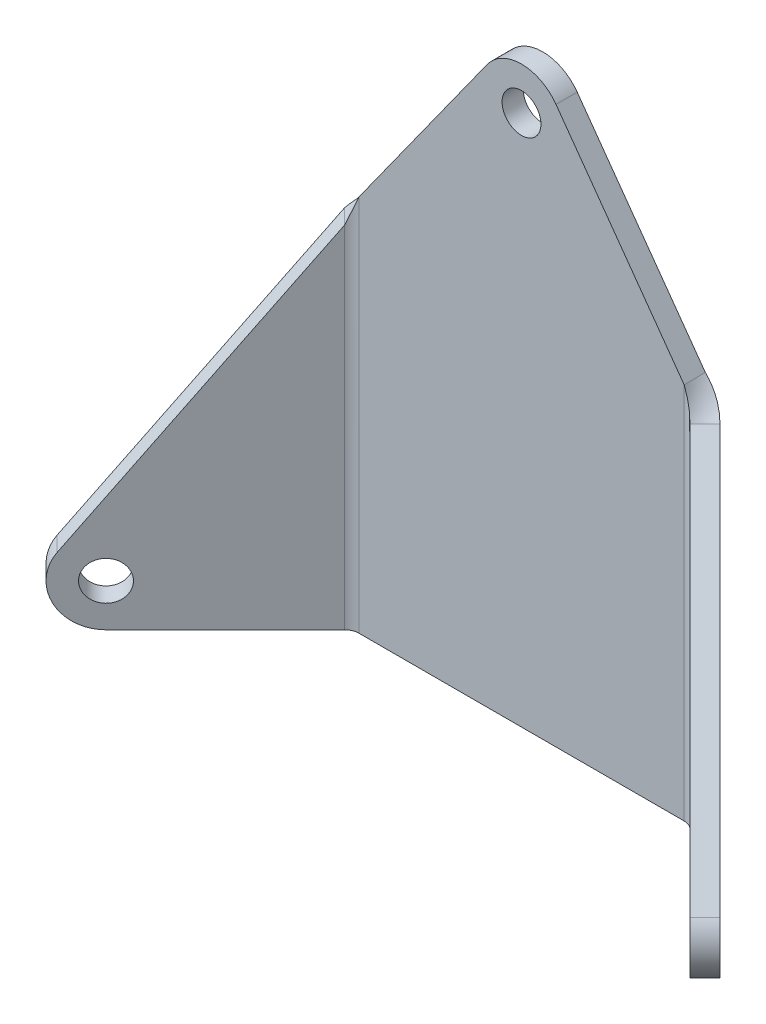
ISO-10303-21;
HEADER;
FILE_DESCRIPTION(('STEP AP214'),'2;1');
FILE_NAME('part.step','',(''),(''),'','','');
FILE_SCHEMA(('AUTOMOTIVE_DESIGN { 1 0 10303 214 1 1 1 1 }'));
ENDSEC;
DATA;
#1=APPLICATION_CONTEXT('core data for automotive mechanical design processes');
#2=APPLICATION_PROTOCOL_DEFINITION('international standard','automotive_design',2000,#1);
#3=PRODUCT_CONTEXT('',#1,'mechanical');
#4=PRODUCT('Part','Part','',(#3));
#5=PRODUCT_RELATED_PRODUCT_CATEGORY('part','',(#4));
#6=PRODUCT_DEFINITION_FORMATION('','',#4);
#7=PRODUCT_DEFINITION_CONTEXT('part definition',#1,'design');
#8=PRODUCT_DEFINITION('design','',#6,#7);
#9=PRODUCT_DEFINITION_SHAPE('','',#8);
#10=(LENGTH_UNIT() NAMED_UNIT(*) SI_UNIT(.MILLI.,.METRE.));
#11=(NAMED_UNIT(*) PLANE_ANGLE_UNIT() SI_UNIT($,.RADIAN.));
#12=(NAMED_UNIT(*) SI_UNIT($,.STERADIAN.) SOLID_ANGLE_UNIT());
#13=UNCERTAINTY_MEASURE_WITH_UNIT(LENGTH_MEASURE(1.E-05),#10,'distance_accuracy_value','');
#14=(GEOMETRIC_REPRESENTATION_CONTEXT(3) GLOBAL_UNCERTAINTY_ASSIGNED_CONTEXT((#13)) GLOBAL_UNIT_ASSIGNED_CONTEXT((#10,
#11,#12)) REPRESENTATION_CONTEXT('',''));
#15=CARTESIAN_POINT('',(0.,0.,0.));
#16=DIRECTION('',(0.,0.,1.));
#17=DIRECTION('',(1.,0.,0.));
#18=AXIS2_PLACEMENT_3D('',#15,#16,#17);
#19=CARTESIAN_POINT('',(346.082397664903,60.300507275373,-19.05));
#20=DIRECTION('',(0.812694164433091,0.58269047966858,0.));
#21=DIRECTION('',(-0.58269047966858,0.812694164433091,0.));
#22=AXIS2_PLACEMENT_3D('',#19,#20,#21);
#23=PLANE('',#22);
#24=DIRECTION('',(-0.58269047966858,0.812694164433091,0.));
#25=VECTOR('',#24,1.);
#26=CARTESIAN_POINT('',(346.082397664903,60.300507275373,0.));
#27=LINE('',#26,#25);
#28=CARTESIAN_POINT('',(146.053512909248,339.28620041977,0.));
#29=VERTEX_POINT('',#28);
#30=CARTESIAN_POINT('',(30.963647664901,499.805146812495,0.));
#31=VERTEX_POINT('',#30);
#32=EDGE_CURVE('E381',#29,#31,#27,.T.);
#33=ORIENTED_EDGE('',*,*,#32,.F.);
#34=CARTESIAN_POINT('',(146.053512909248,339.28620041977,-19.05));
#35=CARTESIAN_POINT('',(146.053512909248,339.28620041977,0.));
#36=B_SPLINE_CURVE_WITH_KNOTS('',1,(#34,#35),.UNSPECIFIED.,.F.,.F.,(2,2),(0.,1.),.UNSPECIFIED.);
#37=CARTESIAN_POINT('',(146.053512909248,339.28620041977,-19.05));
#38=VERTEX_POINT('',#37);
#39=EDGE_CURVE('E283',#29,#38,#36,.F.);
#40=ORIENTED_EDGE('',*,*,#39,.T.);
#41=DIRECTION('',(-0.58269047966858,0.812694164433091,0.));
#42=VECTOR('',#41,1.);
#43=CARTESIAN_POINT('',(346.082397664903,60.300507275373,-19.05));
#44=LINE('',#43,#42);
#45=CARTESIAN_POINT('',(30.963647664901,499.805146812495,-19.05));
#46=VERTEX_POINT('',#45);
#47=EDGE_CURVE('E396',#38,#46,#44,.T.);
#48=ORIENTED_EDGE('',*,*,#47,.T.);
#49=DIRECTION('',(0.,0.,1.));
#50=VECTOR('',#49,1.);
#51=CARTESIAN_POINT('',(30.963647664901,499.805146812495,-19.05));
#52=LINE('',#51,#50);
#53=EDGE_CURVE('E393',#46,#31,#52,.T.);
#54=ORIENTED_EDGE('',*,*,#53,.T.);
#55=EDGE_LOOP('',(#33,#40,#48,#54));
#56=FACE_BOUND('',#55,.T.);
#57=ADVANCED_FACE('F65',(#56),#23,.T.);
#58=CARTESIAN_POINT('',(2.77555756156289E-13,477.604639537122,-19.05));
#59=DIRECTION('',(0.,0.,-1.));
#60=DIRECTION('',(-1.,0.,0.));
#61=AXIS2_PLACEMENT_3D('',#58,#59,#60);
#62=PLANE('',#61);
#63=CARTESIAN_POINT('',(2.77555756156289E-13,477.604639537122,-19.05));
#64=DIRECTION('',(0.,0.,1.));
#65=DIRECTION('',(1.,0.,0.));
#66=AXIS2_PLACEMENT_3D('',#63,#64,#65);
#67=CIRCLE('',#66,17.4625);
#68=CARTESIAN_POINT('',(17.4625000000003,477.604639537122,-19.05));
#69=VERTEX_POINT('',#68);
#70=EDGE_CURVE('E383',#69,#69,#67,.T.);
#71=ORIENTED_EDGE('',*,*,#70,.T.);
#72=EDGE_LOOP('',(#71));
#73=FACE_BOUND('',#72,.T.);
#74=ORIENTED_EDGE('',*,*,#47,.F.);
#75=DIRECTION('',(0.,-1.,0.));
#76=VECTOR('',#75,1.);
#77=CARTESIAN_POINT('',(146.053512909248,477.604639537122,-19.05));
#78=LINE('',#77,#76);
#79=CARTESIAN_POINT('',(146.053512909248,0.,-19.05));
#80=VERTEX_POINT('',#79);
#81=EDGE_CURVE('E481',#38,#80,#78,.T.);
#82=ORIENTED_EDGE('',*,*,#81,.T.);
#83=DIRECTION('',(1.,0.,0.));
#84=VECTOR('',#83,1.);
#85=CARTESIAN_POINT('',(-315.118749999997,0.,-19.05));
#86=LINE('',#85,#84);
#87=CARTESIAN_POINT('',(-146.053512909243,0.,-19.05));
#88=VERTEX_POINT('',#87);
#89=EDGE_CURVE('E384',#88,#80,#86,.T.);
#90=ORIENTED_EDGE('',*,*,#89,.F.);
#91=DIRECTION('',(0.,-1.,0.));
#92=VECTOR('',#91,1.);
#93=CARTESIAN_POINT('',(-146.053512909243,477.604639537122,-19.05));
#94=LINE('',#93,#92);
#95=CARTESIAN_POINT('',(-146.053512909243,339.286200419774,-19.05));
#96=VERTEX_POINT('',#95);
#97=EDGE_CURVE('E295',#96,#88,#94,.T.);
#98=ORIENTED_EDGE('',*,*,#97,.F.);
#99=DIRECTION('',(-0.582690479668574,-0.812694164433095,0.));
#100=VECTOR('',#99,1.);
#101=CARTESIAN_POINT('',(-346.082397664898,60.3005072753726,-19.05));
#102=LINE('',#101,#100);
#103=CARTESIAN_POINT('',(-30.9636476649007,499.805146812495,-19.05));
#104=VERTEX_POINT('',#103);
#105=EDGE_CURVE('E390',#104,#96,#102,.T.);
#106=ORIENTED_EDGE('',*,*,#105,.F.);
#107=CARTESIAN_POINT('',(2.77555756156289E-13,477.604639537122,-19.05));
#108=DIRECTION('',(0.,0.,1.));
#109=DIRECTION('',(-1.,0.,0.));
#110=AXIS2_PLACEMENT_3D('',#107,#108,#109);
#111=CIRCLE('',#110,38.1);
#112=EDGE_CURVE('E391',#46,#104,#111,.T.);
#113=ORIENTED_EDGE('',*,*,#112,.F.);
#114=EDGE_LOOP('',(#74,#82,#90,#98,#106,#113));
#115=FACE_BOUND('',#114,.T.);
#116=ADVANCED_FACE('F510',(#73,#115),#62,.T.);
#117=CARTESIAN_POINT('',(-315.118749999997,0.,-19.05));
#118=DIRECTION('',(0.,-1.,0.));
#119=DIRECTION('',(1.,0.,0.));
#120=AXIS2_PLACEMENT_3D('',#117,#118,#119);
#121=PLANE('',#120);
#122=ORIENTED_EDGE('',*,*,#89,.T.);
#123=DIRECTION('',(0.,0.,1.));
#124=VECTOR('',#123,1.);
#125=CARTESIAN_POINT('',(146.053512909248,0.,-19.05));
#126=LINE('',#125,#124);
#127=CARTESIAN_POINT('',(146.053512909248,0.,0.));
#128=VERTEX_POINT('',#127);
#129=EDGE_CURVE('E12',#80,#128,#126,.T.);
#130=ORIENTED_EDGE('',*,*,#129,.T.);
#131=DIRECTION('',(1.,0.,0.));
#132=VECTOR('',#131,1.);
#133=CARTESIAN_POINT('',(-315.118749999997,0.,0.));
#134=LINE('',#133,#132);
#135=CARTESIAN_POINT('',(-146.053512909243,0.,0.));
#136=VERTEX_POINT('',#135);
#137=EDGE_CURVE('E479',#136,#128,#134,.T.);
#138=ORIENTED_EDGE('',*,*,#137,.F.);
#139=DIRECTION('',(0.,0.,1.));
#140=VECTOR('',#139,1.);
#141=CARTESIAN_POINT('',(-146.053512909243,0.,-19.05));
#142=LINE('',#141,#140);
#143=EDGE_CURVE('E402',#88,#136,#142,.T.);
#144=ORIENTED_EDGE('',*,*,#143,.F.);
#145=EDGE_LOOP('',(#122,#130,#138,#144));
#146=FACE_BOUND('',#145,.T.);
#147=ADVANCED_FACE('F62',(#146),#121,.T.);
#148=CARTESIAN_POINT('',(-275.708444659128,0.,97.4536511445398));
#149=DIRECTION('',(0.,-1.,0.));
#150=DIRECTION('',(0.707106781186546,0.,-0.707106781186549));
#151=AXIS2_PLACEMENT_3D('',#148,#149,#150);
#152=PLANE('',#151);
#153=DIRECTION('',(0.707106781186546,0.,-0.707106781186549));
#154=VECTOR('',#153,1.);
#155=CARTESIAN_POINT('',(-275.708444659128,0.,97.4536511445398));
#156=LINE('',#155,#154);
#157=CARTESIAN_POINT('',(-275.708444659128,0.,97.4536511445398));
#158=VERTEX_POINT('',#157);
#159=CARTESIAN_POINT('',(-168.504153211916,0.,-9.75064030267285));
#160=VERTEX_POINT('',#159);
#161=EDGE_CURVE('E550',#158,#160,#156,.T.);
#162=ORIENTED_EDGE('',*,*,#161,.T.);
#163=DIRECTION('',(0.707106781186549,0.,0.707106781186546));
#164=VECTOR('',#163,1.);
#165=CARTESIAN_POINT('',(-168.504153211916,0.,-9.75064030267285));
#166=LINE('',#165,#164);
#167=CARTESIAN_POINT('',(-155.033769030312,0.,3.71974387893086));
#168=VERTEX_POINT('',#167);
#169=EDGE_CURVE('E473',#160,#168,#166,.T.);
#170=ORIENTED_EDGE('',*,*,#169,.T.);
#171=DIRECTION('',(0.707106781186546,0.,-0.707106781186549));
#172=VECTOR('',#171,1.);
#173=CARTESIAN_POINT('',(-262.238060477525,0.,110.924035326143));
#174=LINE('',#173,#172);
#175=CARTESIAN_POINT('',(-262.238060477525,0.,110.924035326143));
#176=VERTEX_POINT('',#175);
#177=EDGE_CURVE('E538',#176,#168,#174,.T.);
#178=ORIENTED_EDGE('',*,*,#177,.F.);
#179=DIRECTION('',(0.707106781186549,0.,0.707106781186546));
#180=VECTOR('',#179,1.);
#181=CARTESIAN_POINT('',(-275.708444659128,0.,97.4536511445398));
#182=LINE('',#181,#180);
#183=EDGE_CURVE('E560',#158,#176,#182,.T.);
#184=ORIENTED_EDGE('',*,*,#183,.F.);
#185=EDGE_LOOP('',(#162,#170,#178,#184));
#186=FACE_BOUND('',#185,.T.);
#187=ADVANCED_FACE('F451',(#186),#152,.T.);
#188=CARTESIAN_POINT('',(-297.603049893251,60.3005072753727,119.348256378662));
#189=DIRECTION('',(-0.574661554701376,0.582690479668574,0.574661554701378));
#190=DIRECTION('',(-0.41202438950649,-0.812694164433096,0.412024389506492));
#191=AXIS2_PLACEMENT_3D('',#188,#189,#190);
#192=PLANE('',#191);
#193=DIRECTION('',(-0.41202438950649,-0.812694164433095,0.412024389506492));
#194=VECTOR('',#193,1.);
#195=CARTESIAN_POINT('',(-284.132665711647,60.3005072753727,132.818640560266));
#196=LINE('',#195,#194);
#197=CARTESIAN_POINT('',(-155.033769030312,314.940578687988,3.71974387893086));
#198=VERTEX_POINT('',#197);
#199=CARTESIAN_POINT('',(-284.132665711647,60.3005072753727,132.818640560266));
#200=VERTEX_POINT('',#199);
#201=EDGE_CURVE('E464',#198,#200,#196,.T.);
#202=ORIENTED_EDGE('',*,*,#201,.F.);
#203=CARTESIAN_POINT('',(-168.504153211916,314.940578687988,-9.75064030267285));
#204=CARTESIAN_POINT('',(-155.033769030312,314.940578687988,3.71974387893086));
#205=B_SPLINE_CURVE_WITH_KNOTS('',1,(#203,#204),.UNSPECIFIED.,.F.,.F.,(2,2),(0.,1.),.UNSPECIFIED.);
#206=CARTESIAN_POINT('',(-168.504153211916,314.940578687988,-9.75064030267284));
#207=VERTEX_POINT('',#206);
#208=EDGE_CURVE('E371',#198,#207,#205,.F.);
#209=ORIENTED_EDGE('',*,*,#208,.T.);
#210=DIRECTION('',(-0.41202438950649,-0.812694164433095,0.412024389506492));
#211=VECTOR('',#210,1.);
#212=CARTESIAN_POINT('',(-297.603049893251,60.3005072753727,119.348256378662));
#213=LINE('',#212,#211);
#214=CARTESIAN_POINT('',(-297.603049893251,60.3005072753727,119.348256378662));
#215=VERTEX_POINT('',#214);
#216=EDGE_CURVE('E542',#207,#215,#213,.T.);
#217=ORIENTED_EDGE('',*,*,#216,.T.);
#218=DIRECTION('',(0.707106781186549,0.,0.707106781186546));
#219=VECTOR('',#218,1.);
#220=CARTESIAN_POINT('',(-297.603049893251,60.3005072753727,119.348256378662));
#221=LINE('',#220,#219);
#222=EDGE_CURVE('E553',#215,#200,#221,.T.);
#223=ORIENTED_EDGE('',*,*,#222,.T.);
#224=EDGE_LOOP('',(#202,#209,#217,#223));
#225=FACE_BOUND('',#224,.T.);
#226=ADVANCED_FACE('F450',(#225),#192,.T.);
#227=CARTESIAN_POINT('',(-52.8858396551021,477.604639537122,-125.368953859487));
#228=DIRECTION('',(-0.707106781186549,0.,-0.707106781186546));
#229=DIRECTION('',(-0.707106781186546,0.,0.707106781186549));
#230=AXIS2_PLACEMENT_3D('',#227,#228,#229);
#231=PLANE('',#230);
#232=CARTESIAN_POINT('',(-275.708444659128,38.1,97.4536511445398));
#233=DIRECTION('',(0.707106781186549,0.,0.707106781186546));
#234=DIRECTION('',(0.707106781186546,0.,-0.707106781186549));
#235=AXIS2_PLACEMENT_3D('',#232,#233,#234);
#236=CIRCLE('',#235,17.4625);
#237=CARTESIAN_POINT('',(-263.360592492658,38.1,85.1057989780697));
#238=VERTEX_POINT('',#237);
#239=EDGE_CURVE('E469',#238,#238,#236,.T.);
#240=ORIENTED_EDGE('',*,*,#239,.T.);
#241=EDGE_LOOP('',(#240));
#242=FACE_BOUND('',#241,.T.);
#243=ORIENTED_EDGE('',*,*,#216,.F.);
#244=DIRECTION('',(0.,-1.,0.));
#245=VECTOR('',#244,1.);
#246=CARTESIAN_POINT('',(-168.504153211916,477.604639537122,-9.75064030267284));
#247=LINE('',#246,#245);
#248=EDGE_CURVE('E554',#207,#160,#247,.T.);
#249=ORIENTED_EDGE('',*,*,#248,.T.);
#250=ORIENTED_EDGE('',*,*,#161,.F.);
#251=CARTESIAN_POINT('',(-275.708444659128,38.1,97.4536511445398));
#252=DIRECTION('',(0.707106781186549,0.,0.707106781186546));
#253=DIRECTION('',(-0.707106781186546,0.,0.707106781186549));
#254=AXIS2_PLACEMENT_3D('',#251,#252,#253);
#255=CIRCLE('',#254,38.1);
#256=EDGE_CURVE('E551',#215,#158,#255,.T.);
#257=ORIENTED_EDGE('',*,*,#256,.F.);
#258=EDGE_LOOP('',(#243,#249,#250,#257));
#259=FACE_BOUND('',#258,.T.);
#260=ADVANCED_FACE('F442',(#242,#259),#231,.T.);
#261=CARTESIAN_POINT('',(-275.708444659128,38.1,97.4536511445398));
#262=DIRECTION('',(0.707106781186549,0.,0.707106781186546));
#263=DIRECTION('',(0.707106781186546,0.,-0.707106781186549));
#264=AXIS2_PLACEMENT_3D('',#261,#262,#263);
#265=CYLINDRICAL_SURFACE('',#264,38.1);
#266=CARTESIAN_POINT('',(-262.238060477525,38.1,110.924035326143));
#267=DIRECTION('',(0.707106781186549,0.,0.707106781186546));
#268=DIRECTION('',(-0.707106781186546,0.,0.707106781186549));
#269=AXIS2_PLACEMENT_3D('',#266,#267,#268);
#270=CIRCLE('',#269,38.1);
#271=EDGE_CURVE('E466',#200,#176,#270,.T.);
#272=ORIENTED_EDGE('',*,*,#271,.F.);
#273=ORIENTED_EDGE('',*,*,#222,.F.);
#274=ORIENTED_EDGE('',*,*,#256,.T.);
#275=ORIENTED_EDGE('',*,*,#183,.T.);
#276=EDGE_LOOP('',(#272,#273,#274,#275));
#277=FACE_BOUND('',#276,.T.);
#278=ADVANCED_FACE('F439',(#277),#265,.T.);
#279=CARTESIAN_POINT('',(-39.4154554734983,477.604639537122,-111.898569677884));
#280=DIRECTION('',(-0.707106781186549,0.,-0.707106781186546));
#281=DIRECTION('',(-0.707106781186546,0.,0.707106781186549));
#282=AXIS2_PLACEMENT_3D('',#279,#280,#281);
#283=PLANE('',#282);
#284=DIRECTION('',(0.,-1.,0.));
#285=VECTOR('',#284,1.);
#286=CARTESIAN_POINT('',(-155.033769030312,477.604639537122,3.71974387893087));
#287=LINE('',#286,#285);
#288=EDGE_CURVE('E471',#198,#168,#287,.T.);
#289=ORIENTED_EDGE('',*,*,#288,.F.);
#290=ORIENTED_EDGE('',*,*,#201,.T.);
#291=ORIENTED_EDGE('',*,*,#271,.T.);
#292=ORIENTED_EDGE('',*,*,#177,.T.);
#293=EDGE_LOOP('',(#289,#290,#291,#292));
#294=FACE_BOUND('',#293,.T.);
#295=CARTESIAN_POINT('',(-262.238060477525,38.1,110.924035326143));
#296=DIRECTION('',(0.707106781186549,0.,0.707106781186546));
#297=DIRECTION('',(0.707106781186546,0.,-0.707106781186549));
#298=AXIS2_PLACEMENT_3D('',#295,#296,#297);
#299=CIRCLE('',#298,17.4625);
#300=CARTESIAN_POINT('',(-249.890208311054,38.1,98.5761831596734));
#301=VERTEX_POINT('',#300);
#302=EDGE_CURVE('E478',#301,#301,#299,.T.);
#303=ORIENTED_EDGE('',*,*,#302,.F.);
#304=EDGE_LOOP('',(#303));
#305=FACE_BOUND('',#304,.T.);
#306=ADVANCED_FACE('F438',(#294,#305),#283,.F.);
#307=CARTESIAN_POINT('',(-275.708444659128,38.1,97.4536511445398));
#308=DIRECTION('',(0.707106781186549,0.,0.707106781186546));
#309=DIRECTION('',(0.707106781186546,0.,-0.707106781186549));
#310=AXIS2_PLACEMENT_3D('',#307,#308,#309);
#311=CYLINDRICAL_SURFACE('',#310,17.4625);
#312=ORIENTED_EDGE('',*,*,#239,.F.);
#313=EDGE_LOOP('',(#312));
#314=FACE_BOUND('',#313,.T.);
#315=ORIENTED_EDGE('',*,*,#302,.T.);
#316=EDGE_LOOP('',(#315));
#317=FACE_BOUND('',#316,.T.);
#318=ADVANCED_FACE('F432',(#314,#317),#311,.F.);
#319=CARTESIAN_POINT('',(2.77555756156289E-13,477.604639537122,-19.05));
#320=DIRECTION('',(0.,0.,1.));
#321=DIRECTION('',(1.,0.,0.));
#322=AXIS2_PLACEMENT_3D('',#319,#320,#321);
#323=CYLINDRICAL_SURFACE('',#322,17.4625);
#324=CARTESIAN_POINT('',(2.77555756156289E-13,477.604639537122,0.));
#325=DIRECTION('',(0.,0.,1.));
#326=DIRECTION('',(1.,0.,0.));
#327=AXIS2_PLACEMENT_3D('',#324,#325,#326);
#328=CIRCLE('',#327,17.4625);
#329=CARTESIAN_POINT('',(17.4625000000003,477.604639537122,0.));
#330=VERTEX_POINT('',#329);
#331=EDGE_CURVE('E400',#330,#330,#328,.T.);
#332=CARTESIAN_POINT('',(17.4625000000003,477.604639537122,-19.05));
#333=CARTESIAN_POINT('',(17.4625000000003,477.604639537122,-18.8515625));
#334=CARTESIAN_POINT('',(17.4625000000003,477.604639537122,-18.653125));
#335=CARTESIAN_POINT('',(17.4625000000003,477.604639537122,-18.25625));
#336=CARTESIAN_POINT('',(17.4625000000003,477.604639537122,-18.0578125));
#337=CARTESIAN_POINT('',(17.4625000000003,477.604639537122,-17.6609375));
#338=CARTESIAN_POINT('',(17.4625000000003,477.604639537122,-17.4625));
#339=CARTESIAN_POINT('',(17.4625000000003,477.604639537122,-17.065625));
#340=CARTESIAN_POINT('',(17.4625000000003,477.604639537122,-16.8671875));
#341=CARTESIAN_POINT('',(17.4625000000003,477.604639537122,-16.4703125));
#342=CARTESIAN_POINT('',(17.4625000000003,477.604639537122,-16.271875));
#343=CARTESIAN_POINT('',(17.4625000000003,477.604639537122,-15.875));
#344=CARTESIAN_POINT('',(17.4625000000003,477.604639537122,-15.6765625));
#345=CARTESIAN_POINT('',(17.4625000000003,477.604639537122,-15.2796875));
#346=CARTESIAN_POINT('',(17.4625000000003,477.604639537122,-15.08125));
#347=CARTESIAN_POINT('',(17.4625000000003,477.604639537122,-14.684375));
#348=CARTESIAN_POINT('',(17.4625000000003,477.604639537122,-14.4859375));
#349=CARTESIAN_POINT('',(17.4625000000003,477.604639537122,-14.0890625));
#350=CARTESIAN_POINT('',(17.4625000000003,477.604639537122,-13.890625));
#351=CARTESIAN_POINT('',(17.4625000000003,477.604639537122,-13.49375));
#352=CARTESIAN_POINT('',(17.4625000000003,477.604639537122,-13.2953125));
#353=CARTESIAN_POINT('',(17.4625000000003,477.604639537122,-12.8984375));
#354=CARTESIAN_POINT('',(17.4625000000003,477.604639537122,-12.7));
#355=CARTESIAN_POINT('',(17.4625000000003,477.604639537122,-12.303125));
#356=CARTESIAN_POINT('',(17.4625000000003,477.604639537122,-12.1046875));
#357=CARTESIAN_POINT('',(17.4625000000003,477.604639537122,-11.7078125));
#358=CARTESIAN_POINT('',(17.4625000000003,477.604639537122,-11.509375));
#359=CARTESIAN_POINT('',(17.4625000000003,477.604639537122,-11.1125));
#360=CARTESIAN_POINT('',(17.4625000000003,477.604639537122,-10.9140625));
#361=CARTESIAN_POINT('',(17.4625000000003,477.604639537122,-10.5171875));
#362=CARTESIAN_POINT('',(17.4625000000003,477.604639537122,-10.31875));
#363=CARTESIAN_POINT('',(17.4625000000003,477.604639537122,-9.921875));
#364=CARTESIAN_POINT('',(17.4625000000003,477.604639537122,-9.7234375));
#365=CARTESIAN_POINT('',(17.4625000000003,477.604639537122,-9.3265625));
#366=CARTESIAN_POINT('',(17.4625000000003,477.604639537122,-9.128125));
#367=CARTESIAN_POINT('',(17.4625000000003,477.604639537122,-8.73125));
#368=CARTESIAN_POINT('',(17.4625000000003,477.604639537122,-8.5328125));
#369=CARTESIAN_POINT('',(17.4625000000003,477.604639537122,-8.1359375));
#370=CARTESIAN_POINT('',(17.4625000000003,477.604639537122,-7.9375));
#371=CARTESIAN_POINT('',(17.4625000000003,477.604639537122,-7.540625));
#372=CARTESIAN_POINT('',(17.4625000000003,477.604639537122,-7.3421875));
#373=CARTESIAN_POINT('',(17.4625000000003,477.604639537122,-6.9453125));
#374=CARTESIAN_POINT('',(17.4625000000003,477.604639537122,-6.746875));
#375=CARTESIAN_POINT('',(17.4625000000003,477.604639537122,-6.35));
#376=CARTESIAN_POINT('',(17.4625000000003,477.604639537122,-6.1515625));
#377=CARTESIAN_POINT('',(17.4625000000003,477.604639537122,-5.7546875));
#378=CARTESIAN_POINT('',(17.4625000000003,477.604639537122,-5.55625));
#379=CARTESIAN_POINT('',(17.4625000000003,477.604639537122,-5.159375));
#380=CARTESIAN_POINT('',(17.4625000000003,477.604639537122,-4.9609375));
#381=CARTESIAN_POINT('',(17.4625000000003,477.604639537122,-4.5640625));
#382=CARTESIAN_POINT('',(17.4625000000003,477.604639537122,-4.365625));
#383=CARTESIAN_POINT('',(17.4625000000003,477.604639537122,-3.96875));
#384=CARTESIAN_POINT('',(17.4625000000003,477.604639537122,-3.7703125));
#385=CARTESIAN_POINT('',(17.4625000000003,477.604639537122,-3.3734375));
#386=CARTESIAN_POINT('',(17.4625000000003,477.604639537122,-3.175));
#387=CARTESIAN_POINT('',(17.4625000000003,477.604639537122,-2.778125));
#388=CARTESIAN_POINT('',(17.4625000000003,477.604639537122,-2.5796875));
#389=CARTESIAN_POINT('',(17.4625000000003,477.604639537122,-2.1828125));
#390=CARTESIAN_POINT('',(17.4625000000003,477.604639537122,-1.984375));
#391=CARTESIAN_POINT('',(17.4625000000003,477.604639537122,-1.5875));
#392=CARTESIAN_POINT('',(17.4625000000003,477.604639537122,-1.3890625));
#393=CARTESIAN_POINT('',(17.4625000000003,477.604639537122,-0.992187500000001));
#394=CARTESIAN_POINT('',(17.4625000000003,477.604639537122,-0.793750000000001));
#395=CARTESIAN_POINT('',(17.4625000000003,477.604639537122,-0.396875));
#396=CARTESIAN_POINT('',(17.4625000000003,477.604639537122,-0.1984375));
#397=CARTESIAN_POINT('',(17.4625000000003,477.604639537122,0.));
#398=B_SPLINE_CURVE_WITH_KNOTS('',3,(#332,#333,#334,#335,#336,#337,#338,#339,#340,#341,#342,
#343,#344,#345,#346,#347,#348,#349,#350,#351,#352,#353,#354,#355,#356,#357,#358,#359,#360,#361,
#362,#363,#364,#365,#366,#367,#368,#369,#370,#371,#372,#373,#374,#375,#376,#377,#378,#379,#380,
#381,#382,#383,#384,#385,#386,#387,#388,#389,#390,#391,#392,#393,#394,#395,#396,#397),
.UNSPECIFIED.,.F.,.F.,(4,2,2,2,2,2,2,2,2,2,2,2,2,2,2,2,2,2,2,2,2,2,2,2,2,2,2,2,2,2,2,2,4),(0.,
0.5953125,1.190625,1.7859375,2.38125,2.9765625,3.571875,4.1671875,4.7625,5.3578125,5.953125,
6.5484375,7.14375,7.7390625,8.334375,8.9296875,9.525,10.1203125,10.715625,11.3109375,11.90625,
12.5015625,13.096875,13.6921875,14.2875,14.8828125,15.478125,16.0734375,16.66875,17.2640625,
17.859375,18.4546875,19.05),.UNSPECIFIED.);
#399=EDGE_CURVE('BSEAM440',#69,#330,#398,.T.);
#400=ORIENTED_EDGE('',*,*,#70,.F.);
#401=ORIENTED_EDGE('',*,*,#331,.T.);
#402=ORIENTED_EDGE('',*,*,#399,.T.);
#403=ORIENTED_EDGE('',*,*,#399,.F.);
#404=EDGE_LOOP('',(#400,#402,#401,#403));
#405=FACE_BOUND('',#404,.T.);
#406=ADVANCED_FACE('F440',(#405),#323,.F.);
#407=CARTESIAN_POINT('',(2.77555756156289E-13,477.604639537122,-19.05));
#408=DIRECTION('',(0.,0.,1.));
#409=DIRECTION('',(1.,0.,0.));
#410=AXIS2_PLACEMENT_3D('',#407,#408,#409);
#411=CYLINDRICAL_SURFACE('',#410,38.1);
#412=CARTESIAN_POINT('',(2.77555756156289E-13,477.604639537122,0.));
#413=DIRECTION('',(0.,0.,1.));
#414=DIRECTION('',(-1.,0.,0.));
#415=AXIS2_PLACEMENT_3D('',#412,#413,#414);
#416=CIRCLE('',#415,38.1);
#417=CARTESIAN_POINT('',(-30.9636476649007,499.805146812495,0.));
#418=VERTEX_POINT('',#417);
#419=EDGE_CURVE('E374',#31,#418,#416,.T.);
#420=ORIENTED_EDGE('',*,*,#419,.F.);
#421=ORIENTED_EDGE('',*,*,#53,.F.);
#422=ORIENTED_EDGE('',*,*,#112,.T.);
#423=DIRECTION('',(0.,0.,1.));
#424=VECTOR('',#423,1.);
#425=CARTESIAN_POINT('',(-30.9636476649007,499.805146812495,-19.05));
#426=LINE('',#425,#424);
#427=EDGE_CURVE('E388',#104,#418,#426,.T.);
#428=ORIENTED_EDGE('',*,*,#427,.T.);
#429=EDGE_LOOP('',(#420,#421,#422,#428));
#430=FACE_BOUND('',#429,.T.);
#431=ADVANCED_FACE('F435',(#430),#411,.T.);
#432=CARTESIAN_POINT('',(-346.082397664898,60.3005072753726,-19.05));
#433=DIRECTION('',(-0.812694164433095,0.582690479668574,0.));
#434=DIRECTION('',(-0.582690479668574,-0.812694164433096,0.));
#435=AXIS2_PLACEMENT_3D('',#432,#433,#434);
#436=PLANE('',#435);
#437=CARTESIAN_POINT('',(-146.053512909243,339.286200419774,0.));
#438=CARTESIAN_POINT('',(-146.053512909243,339.286200419774,-19.05));
#439=B_SPLINE_CURVE_WITH_KNOTS('',1,(#437,#438),.UNSPECIFIED.,.F.,.F.,(2,2),(0.,1.),.UNSPECIFIED.);
#440=CARTESIAN_POINT('',(-146.053512909243,339.286200419774,0.));
#441=VERTEX_POINT('',#440);
#442=EDGE_CURVE('E359',#441,#96,#439,.T.);
#443=ORIENTED_EDGE('',*,*,#442,.F.);
#444=DIRECTION('',(-0.582690479668574,-0.812694164433095,0.));
#445=VECTOR('',#444,1.);
#446=CARTESIAN_POINT('',(-346.082397664898,60.3005072753726,0.));
#447=LINE('',#446,#445);
#448=EDGE_CURVE('E403',#418,#441,#447,.T.);
#449=ORIENTED_EDGE('',*,*,#448,.F.);
#450=ORIENTED_EDGE('',*,*,#427,.F.);
#451=ORIENTED_EDGE('',*,*,#105,.T.);
#452=EDGE_LOOP('',(#443,#449,#450,#451));
#453=FACE_BOUND('',#452,.T.);
#454=ADVANCED_FACE('F423',(#453),#436,.T.);
#455=CARTESIAN_POINT('',(2.77555756156289E-13,477.604639537122,0.));
#456=DIRECTION('',(0.,0.,-1.));
#457=DIRECTION('',(-1.,0.,0.));
#458=AXIS2_PLACEMENT_3D('',#455,#456,#457);
#459=PLANE('',#458);
#460=DIRECTION('',(0.,-1.,0.));
#461=VECTOR('',#460,1.);
#462=CARTESIAN_POINT('',(146.053512909248,477.604639537122,0.));
#463=LINE('',#462,#461);
#464=EDGE_CURVE('E71',#29,#128,#463,.T.);
#465=ORIENTED_EDGE('',*,*,#464,.F.);
#466=ORIENTED_EDGE('',*,*,#32,.T.);
#467=ORIENTED_EDGE('',*,*,#419,.T.);
#468=ORIENTED_EDGE('',*,*,#448,.T.);
#469=DIRECTION('',(0.,-1.,0.));
#470=VECTOR('',#469,1.);
#471=CARTESIAN_POINT('',(-146.053512909243,477.604639537122,0.));
#472=LINE('',#471,#470);
#473=EDGE_CURVE('E419',#441,#136,#472,.T.);
#474=ORIENTED_EDGE('',*,*,#473,.T.);
#475=ORIENTED_EDGE('',*,*,#137,.T.);
#476=EDGE_LOOP('',(#465,#466,#467,#468,#474,#475));
#477=FACE_BOUND('',#476,.T.);
#478=ORIENTED_EDGE('',*,*,#331,.F.);
#479=EDGE_LOOP('',(#478));
#480=FACE_BOUND('',#479,.T.);
#481=ADVANCED_FACE('F431',(#477,#480),#459,.F.);
#482=CARTESIAN_POINT('',(-168.504153211916,314.940578687988,-9.75064030267285));
#483=CARTESIAN_POINT('',(-165.565099990519,318.998556865915,-12.6896935240697));
#484=CARTESIAN_POINT('',(-162.043415536019,323.055785931916,-15.0427178302477));
#485=CARTESIAN_POINT('',(-154.36400823765,331.170993175845,-18.223632484219));
#486=CARTESIAN_POINT('',(-150.209961835479,335.228222241847,-19.05));
#487=CARTESIAN_POINT('',(-146.053512909243,339.286200419774,-19.05));
#488=CARTESIAN_POINT('',(-155.033769030312,314.940578687988,3.71974387893086));
#489=CARTESIAN_POINT('',(-153.85822579001,318.998287461028,2.5442006386284));
#490=CARTESIAN_POINT('',(-152.449473959954,323.055785931916,1.60291286790094));
#491=CARTESIAN_POINT('',(-149.377711040606,331.170993175845,0.330547006312403));
#492=CARTESIAN_POINT('',(-147.715982102835,335.228491646734,0.));
#493=CARTESIAN_POINT('',(-146.053512909243,339.286200419774,0.));
#494=B_SPLINE_SURFACE_WITH_KNOTS('',1,3,((#482,#483,#484,#485,#486,#487),(#488,#489,#490,#491,
#492,#493)),.UNSPECIFIED.,.F.,.F.,.F.,(2,2),(4,2,4),(0.,1.),(0.,0.5,1.),.UNSPECIFIED.);
#495=CARTESIAN_POINT('',(-155.033769030312,314.940578687988,3.71974387893086));
#496=CARTESIAN_POINT('',(-153.85822579001,318.998287461028,2.5442006386284));
#497=CARTESIAN_POINT('',(-152.449473959954,323.055785931916,1.60291286790094));
#498=CARTESIAN_POINT('',(-149.377711040606,331.170993175845,0.330547006312403));
#499=CARTESIAN_POINT('',(-147.715982102835,335.228491646734,0.));
#500=CARTESIAN_POINT('',(-146.053512909243,339.286200419774,0.));
#501=B_SPLINE_CURVE_WITH_KNOTS('',3,(#495,#496,#497,#498,#499,#500),.UNSPECIFIED.,.F.,.F.,(4,2,
4),(0.,0.5,1.),.UNSPECIFIED.);
#502=EDGE_CURVE('E207',#198,#441,#501,.T.);
#503=CARTESIAN_POINT('',(-146.053512909243,339.286200419774,-19.05));
#504=CARTESIAN_POINT('',(-150.209961835479,335.228222241847,-19.05));
#505=CARTESIAN_POINT('',(-154.36400823765,331.170993175845,-18.223632484219));
#506=CARTESIAN_POINT('',(-162.043415536019,323.055785931916,-15.0427178302477));
#507=CARTESIAN_POINT('',(-165.565099990519,318.998556865915,-12.6896935240697));
#508=CARTESIAN_POINT('',(-168.504153211916,314.940578687988,-9.75064030267285));
#509=B_SPLINE_CURVE_WITH_KNOTS('',3,(#503,#504,#505,#506,#507,#508),.UNSPECIFIED.,.F.,.F.,(4,2,
4),(0.,0.5,1.),.UNSPECIFIED.);
#510=EDGE_CURVE('E294',#207,#96,#509,.F.);
#511=ORIENTED_EDGE('',*,*,#208,.F.);
#512=ORIENTED_EDGE('',*,*,#502,.T.);
#513=ORIENTED_EDGE('',*,*,#442,.T.);
#514=ORIENTED_EDGE('',*,*,#510,.F.);
#515=EDGE_LOOP('',(#511,#512,#513,#514));
#516=FACE_BOUND('',#515,.T.);
#517=ADVANCED_FACE('F318',(#516),#494,.T.);
#518=CARTESIAN_POINT('',(-146.053512909243,0.,12.7));
#519=DIRECTION('',(0.,-1.,0.));
#520=DIRECTION('',(1.,0.,0.));
#521=AXIS2_PLACEMENT_3D('',#518,#519,#520);
#522=PLANE('',#521);
#523=CARTESIAN_POINT('',(-146.053512909243,0.,12.7));
#524=DIRECTION('',(0.,1.,0.));
#525=DIRECTION('',(-1.,0.,0.));
#526=AXIS2_PLACEMENT_3D('',#523,#524,#525);
#527=CIRCLE('',#526,12.7);
#528=EDGE_CURVE('E298',#136,#168,#527,.T.);
#529=ORIENTED_EDGE('',*,*,#528,.T.);
#530=ORIENTED_EDGE('',*,*,#169,.F.);
#531=CARTESIAN_POINT('',(-146.053512909243,0.,12.7));
#532=DIRECTION('',(0.,1.,0.));
#533=DIRECTION('',(1.,0.,0.));
#534=AXIS2_PLACEMENT_3D('',#531,#532,#533);
#535=CIRCLE('',#534,31.75);
#536=EDGE_CURVE('E87',#88,#160,#535,.T.);
#537=ORIENTED_EDGE('',*,*,#536,.F.);
#538=ORIENTED_EDGE('',*,*,#143,.T.);
#539=EDGE_LOOP('',(#529,#530,#537,#538));
#540=FACE_BOUND('',#539,.T.);
#541=ADVANCED_FACE('F314',(#540),#522,.T.);
#542=CARTESIAN_POINT('',(-146.053512909243,-170.625502329619,12.7));
#543=DIRECTION('',(0.,1.,0.));
#544=DIRECTION('',(-1.,0.,0.));
#545=AXIS2_PLACEMENT_3D('',#542,#543,#544);
#546=CYLINDRICAL_SURFACE('',#545,31.75);
#547=ORIENTED_EDGE('',*,*,#97,.T.);
#548=ORIENTED_EDGE('',*,*,#536,.T.);
#549=ORIENTED_EDGE('',*,*,#248,.F.);
#550=ORIENTED_EDGE('',*,*,#510,.T.);
#551=EDGE_LOOP('',(#547,#548,#549,#550));
#552=FACE_BOUND('',#551,.T.);
#553=ADVANCED_FACE('F304',(#552),#546,.T.);
#554=CARTESIAN_POINT('',(-146.053512909243,-170.625502329619,12.7));
#555=DIRECTION('',(0.,1.,0.));
#556=DIRECTION('',(-1.,0.,0.));
#557=AXIS2_PLACEMENT_3D('',#554,#555,#556);
#558=CYLINDRICAL_SURFACE('',#557,12.7);
#559=ORIENTED_EDGE('',*,*,#473,.F.);
#560=ORIENTED_EDGE('',*,*,#502,.F.);
#561=ORIENTED_EDGE('',*,*,#288,.T.);
#562=ORIENTED_EDGE('',*,*,#528,.F.);
#563=EDGE_LOOP('',(#559,#560,#561,#562));
#564=FACE_BOUND('',#563,.T.);
#565=ADVANCED_FACE('F313',(#564),#558,.F.);
#566=CARTESIAN_POINT('',(146.053512909248,339.28620041977,-19.05));
#567=CARTESIAN_POINT('',(150.209961835484,335.228222241843,-19.05));
#568=CARTESIAN_POINT('',(154.364008237656,331.170993175841,-18.223632484219));
#569=CARTESIAN_POINT('',(162.043415536024,323.055785931913,-15.0427178302477));
#570=CARTESIAN_POINT('',(165.565099990524,318.998556865911,-12.6896935240697));
#571=CARTESIAN_POINT('',(168.504153211921,314.940578687984,-9.75064030267294));
#572=CARTESIAN_POINT('',(146.053512909248,339.28620041977,0.));
#573=CARTESIAN_POINT('',(147.71598210284,335.22849164673,0.));
#574=CARTESIAN_POINT('',(149.377711040611,331.170993175841,0.330547006312389));
#575=CARTESIAN_POINT('',(152.449473959959,323.055785931913,1.60291286790092));
#576=CARTESIAN_POINT('',(153.858225790015,318.998287461024,2.54420063862831));
#577=CARTESIAN_POINT('',(155.033769030318,314.940578687984,3.71974387893082));
#578=B_SPLINE_SURFACE_WITH_KNOTS('',1,3,((#566,#567,#568,#569,#570,#571),(#572,#573,#574,#575,
#576,#577)),.UNSPECIFIED.,.F.,.F.,.F.,(2,2),(4,2,4),(0.,1.),(0.,0.5,1.),.UNSPECIFIED.);
#579=CARTESIAN_POINT('',(146.053512909248,339.28620041977,0.));
#580=CARTESIAN_POINT('',(147.71598210284,335.22849164673,0.));
#581=CARTESIAN_POINT('',(149.377711040611,331.170993175841,0.330547006312389));
#582=CARTESIAN_POINT('',(152.449473959959,323.055785931913,1.60291286790092));
#583=CARTESIAN_POINT('',(153.858225790015,318.998287461024,2.54420063862831));
#584=CARTESIAN_POINT('',(155.033769030318,314.940578687984,3.71974387893082));
#585=B_SPLINE_CURVE_WITH_KNOTS('',3,(#579,#580,#581,#582,#583,#584),.UNSPECIFIED.,.F.,.F.,(4,2,
4),(0.,0.5,1.),.UNSPECIFIED.);
#586=CARTESIAN_POINT('',(155.033769030318,314.940578687984,3.71974387893081));
#587=VERTEX_POINT('',#586);
#588=EDGE_CURVE('E184',#29,#587,#585,.T.);
#589=CARTESIAN_POINT('',(155.033769030318,314.940578687984,3.71974387893082));
#590=CARTESIAN_POINT('',(168.504153211921,314.940578687984,-9.75064030267294));
#591=B_SPLINE_CURVE_WITH_KNOTS('',1,(#589,#590),.UNSPECIFIED.,.F.,.F.,(2,2),(0.,1.),.UNSPECIFIED.);
#592=CARTESIAN_POINT('',(168.504153211921,314.940578687984,-9.75064030267289));
#593=VERTEX_POINT('',#592);
#594=EDGE_CURVE('E197',#587,#593,#591,.T.);
#595=CARTESIAN_POINT('',(168.504153211921,314.940578687984,-9.75064030267294));
#596=CARTESIAN_POINT('',(165.565099990524,318.998556865911,-12.6896935240697));
#597=CARTESIAN_POINT('',(162.043415536024,323.055785931913,-15.0427178302477));
#598=CARTESIAN_POINT('',(154.364008237656,331.170993175841,-18.223632484219));
#599=CARTESIAN_POINT('',(150.209961835484,335.228222241843,-19.05));
#600=CARTESIAN_POINT('',(146.053512909248,339.28620041977,-19.05));
#601=B_SPLINE_CURVE_WITH_KNOTS('',3,(#595,#596,#597,#598,#599,#600),.UNSPECIFIED.,.F.,.F.,(4,2,
4),(0.,0.5,1.),.UNSPECIFIED.);
#602=EDGE_CURVE('E210',#38,#593,#601,.F.);
#603=ORIENTED_EDGE('',*,*,#39,.F.);
#604=ORIENTED_EDGE('',*,*,#588,.T.);
#605=ORIENTED_EDGE('',*,*,#594,.T.);
#606=ORIENTED_EDGE('',*,*,#602,.F.);
#607=EDGE_LOOP('',(#603,#604,#605,#606));
#608=FACE_BOUND('',#607,.T.);
#609=ADVANCED_FACE('F234',(#608),#578,.T.);
#610=CARTESIAN_POINT('',(146.053512909248,0.,12.7));
#611=DIRECTION('',(0.,-1.,0.));
#612=DIRECTION('',(0.,0.,-1.));
#613=AXIS2_PLACEMENT_3D('',#610,#611,#612);
#614=PLANE('',#613);
#615=CARTESIAN_POINT('',(146.053512909248,0.,12.7));
#616=DIRECTION('',(0.,-1.,0.));
#617=DIRECTION('',(0.,0.,-1.));
#618=AXIS2_PLACEMENT_3D('',#615,#616,#617);
#619=CIRCLE('',#618,12.7);
#620=CARTESIAN_POINT('',(155.033769030318,0.,3.71974387893086));
#621=VERTEX_POINT('',#620);
#622=EDGE_CURVE('E78',#621,#128,#619,.F.);
#623=ORIENTED_EDGE('',*,*,#622,.T.);
#624=ORIENTED_EDGE('',*,*,#129,.F.);
#625=CARTESIAN_POINT('',(146.053512909248,0.,12.7));
#626=DIRECTION('',(0.,1.,0.));
#627=DIRECTION('',(0.,0.,-1.));
#628=AXIS2_PLACEMENT_3D('',#625,#626,#627);
#629=CIRCLE('',#628,31.75);
#630=CARTESIAN_POINT('',(168.504153211921,0.,-9.75064030267287));
#631=VERTEX_POINT('',#630);
#632=EDGE_CURVE('E205',#631,#80,#629,.T.);
#633=ORIENTED_EDGE('',*,*,#632,.F.);
#634=DIRECTION('',(-0.707106781186549,0.,0.707106781186546));
#635=VECTOR('',#634,1.);
#636=CARTESIAN_POINT('',(168.504153211921,0.,-9.75064030267285));
#637=LINE('',#636,#635);
#638=EDGE_CURVE('E173',#631,#621,#637,.T.);
#639=ORIENTED_EDGE('',*,*,#638,.T.);
#640=EDGE_LOOP('',(#623,#624,#633,#639));
#641=FACE_BOUND('',#640,.T.);
#642=ADVANCED_FACE('F228',(#641),#614,.T.);
#643=CARTESIAN_POINT('',(146.053512909248,509.911702749387,12.7));
#644=DIRECTION('',(0.,-1.,0.));
#645=DIRECTION('',(0.,0.,-1.));
#646=AXIS2_PLACEMENT_3D('',#643,#644,#645);
#647=CYLINDRICAL_SURFACE('',#646,31.75);
#648=DIRECTION('',(0.,-1.,0.));
#649=VECTOR('',#648,1.);
#650=CARTESIAN_POINT('',(168.504153211921,477.604639537122,-9.75064030267288));
#651=LINE('',#650,#649);
#652=EDGE_CURVE('E201',#593,#631,#651,.T.);
#653=ORIENTED_EDGE('',*,*,#652,.T.);
#654=ORIENTED_EDGE('',*,*,#632,.T.);
#655=ORIENTED_EDGE('',*,*,#81,.F.);
#656=ORIENTED_EDGE('',*,*,#602,.T.);
#657=EDGE_LOOP('',(#653,#654,#655,#656));
#658=FACE_BOUND('',#657,.T.);
#659=ADVANCED_FACE('F212',(#658),#647,.T.);
#660=CARTESIAN_POINT('',(146.053512909248,509.911702749387,12.7));
#661=DIRECTION('',(0.,-1.,0.));
#662=DIRECTION('',(0.,0.,-1.));
#663=AXIS2_PLACEMENT_3D('',#660,#661,#662);
#664=CYLINDRICAL_SURFACE('',#663,12.7);
#665=DIRECTION('',(0.,-1.,0.));
#666=VECTOR('',#665,1.);
#667=CARTESIAN_POINT('',(155.033769030318,477.604639537122,3.71974387893083));
#668=LINE('',#667,#666);
#669=EDGE_CURVE('E827',#587,#621,#668,.T.);
#670=ORIENTED_EDGE('',*,*,#669,.F.);
#671=ORIENTED_EDGE('',*,*,#588,.F.);
#672=ORIENTED_EDGE('',*,*,#464,.T.);
#673=ORIENTED_EDGE('',*,*,#622,.F.);
#674=EDGE_LOOP('',(#670,#671,#672,#673));
#675=FACE_BOUND('',#674,.T.);
#676=ADVANCED_FACE('F222',(#675),#664,.F.);
#677=CARTESIAN_POINT('',(275.708444659134,38.1,97.4536511445398));
#678=DIRECTION('',(-0.707106781186549,0.,0.707106781186546));
#679=DIRECTION('',(0.707106781186546,0.,0.707106781186549));
#680=AXIS2_PLACEMENT_3D('',#677,#678,#679);
#681=CYLINDRICAL_SURFACE('',#680,17.4625000000001);
#682=CARTESIAN_POINT('',(275.708444659134,38.1,97.4536511445398));
#683=DIRECTION('',(-0.707106781186549,0.,0.707106781186546));
#684=DIRECTION('',(0.707106781186546,0.,0.707106781186549));
#685=AXIS2_PLACEMENT_3D('',#682,#683,#684);
#686=CIRCLE('',#685,17.4625000000001);
#687=CARTESIAN_POINT('',(288.056296825604,38.1,109.80150331101));
#688=VERTEX_POINT('',#687);
#689=EDGE_CURVE('E193',#688,#688,#686,.T.);
#690=ORIENTED_EDGE('',*,*,#689,.F.);
#691=EDGE_LOOP('',(#690));
#692=FACE_BOUND('',#691,.T.);
#693=CARTESIAN_POINT('',(262.23806047753,38.1,110.924035326143));
#694=DIRECTION('',(-0.707106781186549,0.,0.707106781186546));
#695=DIRECTION('',(0.707106781186546,0.,0.707106781186549));
#696=AXIS2_PLACEMENT_3D('',#693,#694,#695);
#697=CIRCLE('',#696,17.4625000000001);
#698=CARTESIAN_POINT('',(274.585912644,38.1,123.271887492614));
#699=VERTEX_POINT('',#698);
#700=EDGE_CURVE('E191',#699,#699,#697,.T.);
#701=ORIENTED_EDGE('',*,*,#700,.T.);
#702=EDGE_LOOP('',(#701));
#703=FACE_BOUND('',#702,.T.);
#704=ADVANCED_FACE('F235',(#692,#703),#681,.F.);
#705=CARTESIAN_POINT('',(275.708444659134,38.1,97.4536511445398));
#706=DIRECTION('',(-0.707106781186549,0.,0.707106781186546));
#707=DIRECTION('',(0.707106781186546,0.,0.707106781186549));
#708=AXIS2_PLACEMENT_3D('',#705,#706,#707);
#709=CYLINDRICAL_SURFACE('',#708,38.1);
#710=CARTESIAN_POINT('',(262.23806047753,38.1,110.924035326143));
#711=DIRECTION('',(-0.707106781186549,0.,0.707106781186546));
#712=DIRECTION('',(0.707106781186546,0.,0.707106781186549));
#713=AXIS2_PLACEMENT_3D('',#710,#711,#712);
#714=CIRCLE('',#713,38.1);
#715=CARTESIAN_POINT('',(262.23806047753,0.,110.924035326143));
#716=VERTEX_POINT('',#715);
#717=CARTESIAN_POINT('',(284.132665711652,60.3005072753729,132.818640560266));
#718=VERTEX_POINT('',#717);
#719=EDGE_CURVE('E180',#716,#718,#714,.T.);
#720=ORIENTED_EDGE('',*,*,#719,.F.);
#721=DIRECTION('',(-0.707106781186549,0.,0.707106781186546));
#722=VECTOR('',#721,1.);
#723=CARTESIAN_POINT('',(275.708444659134,0.,97.4536511445398));
#724=LINE('',#723,#722);
#725=CARTESIAN_POINT('',(275.708444659134,0.,97.4536511445398));
#726=VERTEX_POINT('',#725);
#727=EDGE_CURVE('E171',#726,#716,#724,.T.);
#728=ORIENTED_EDGE('',*,*,#727,.F.);
#729=CARTESIAN_POINT('',(275.708444659134,38.1,97.4536511445398));
#730=DIRECTION('',(-0.707106781186549,0.,0.707106781186546));
#731=DIRECTION('',(0.707106781186546,0.,0.707106781186549));
#732=AXIS2_PLACEMENT_3D('',#729,#730,#731);
#733=CIRCLE('',#732,38.1);
#734=CARTESIAN_POINT('',(297.603049893256,60.3005072753729,119.348256378662));
#735=VERTEX_POINT('',#734);
#736=EDGE_CURVE('E185',#726,#735,#733,.T.);
#737=ORIENTED_EDGE('',*,*,#736,.T.);
#738=DIRECTION('',(-0.707106781186549,0.,0.707106781186546));
#739=VECTOR('',#738,1.);
#740=CARTESIAN_POINT('',(297.603049893256,60.3005072753729,119.348256378662));
#741=LINE('',#740,#739);
#742=EDGE_CURVE('E194',#735,#718,#741,.T.);
#743=ORIENTED_EDGE('',*,*,#742,.T.);
#744=EDGE_LOOP('',(#720,#728,#737,#743));
#745=FACE_BOUND('',#744,.T.);
#746=ADVANCED_FACE('F181',(#745),#709,.T.);
#747=CARTESIAN_POINT('',(52.885839655104,477.604639537122,-125.368953859491));
#748=DIRECTION('',(0.707106781186549,0.,-0.707106781186546));
#749=DIRECTION('',(-0.707106781186546,0.,-0.707106781186549));
#750=AXIS2_PLACEMENT_3D('',#747,#748,#749);
#751=PLANE('',#750);
#752=ORIENTED_EDGE('',*,*,#652,.F.);
#753=DIRECTION('',(-0.412024389506494,0.812694164433091,-0.412024389506496));
#754=VECTOR('',#753,1.);
#755=CARTESIAN_POINT('',(297.603049893256,60.300507275373,119.348256378662));
#756=LINE('',#755,#754);
#757=EDGE_CURVE('E188',#735,#593,#756,.T.);
#758=ORIENTED_EDGE('',*,*,#757,.F.);
#759=ORIENTED_EDGE('',*,*,#736,.F.);
#760=DIRECTION('',(0.707106781186546,0.,0.707106781186549));
#761=VECTOR('',#760,1.);
#762=CARTESIAN_POINT('',(-169.936765348922,0.,-348.191558863518));
#763=LINE('',#762,#761);
#764=EDGE_CURVE('E166',#631,#726,#763,.T.);
#765=ORIENTED_EDGE('',*,*,#764,.F.);
#766=EDGE_LOOP('',(#752,#758,#759,#765));
#767=FACE_BOUND('',#766,.T.);
#768=ORIENTED_EDGE('',*,*,#689,.T.);
#769=EDGE_LOOP('',(#768));
#770=FACE_BOUND('',#769,.T.);
#771=ADVANCED_FACE('F190',(#767,#770),#751,.T.);
#772=CARTESIAN_POINT('',(297.603049893256,60.300507275373,119.348256378662));
#773=DIRECTION('',(0.574661554701373,0.58269047966858,0.574661554701375));
#774=DIRECTION('',(-0.412024389506494,0.812694164433091,-0.412024389506496));
#775=AXIS2_PLACEMENT_3D('',#772,#773,#774);
#776=PLANE('',#775);
#777=ORIENTED_EDGE('',*,*,#594,.F.);
#778=DIRECTION('',(-0.412024389506494,0.812694164433091,-0.412024389506496));
#779=VECTOR('',#778,1.);
#780=CARTESIAN_POINT('',(284.132665711652,60.300507275373,132.818640560266));
#781=LINE('',#780,#779);
#782=EDGE_CURVE('E839',#718,#587,#781,.T.);
#783=ORIENTED_EDGE('',*,*,#782,.F.);
#784=ORIENTED_EDGE('',*,*,#742,.F.);
#785=ORIENTED_EDGE('',*,*,#757,.T.);
#786=EDGE_LOOP('',(#777,#783,#784,#785));
#787=FACE_BOUND('',#786,.T.);
#788=ADVANCED_FACE('F722',(#787),#776,.T.);
#789=CARTESIAN_POINT('',(39.4154554735002,477.604639537122,-111.898569677887));
#790=DIRECTION('',(0.707106781186549,0.,-0.707106781186546));
#791=DIRECTION('',(-0.707106781186546,0.,-0.707106781186549));
#792=AXIS2_PLACEMENT_3D('',#789,#790,#791);
#793=PLANE('',#792);
#794=ORIENTED_EDGE('',*,*,#700,.F.);
#795=EDGE_LOOP('',(#794));
#796=FACE_BOUND('',#795,.T.);
#797=ORIENTED_EDGE('',*,*,#782,.T.);
#798=ORIENTED_EDGE('',*,*,#669,.T.);
#799=DIRECTION('',(0.707106781186546,0.,0.707106781186549));
#800=VECTOR('',#799,1.);
#801=CARTESIAN_POINT('',(-183.407149530526,0.,-334.721174681914));
#802=LINE('',#801,#800);
#803=EDGE_CURVE('E840',#621,#716,#802,.T.);
#804=ORIENTED_EDGE('',*,*,#803,.T.);
#805=ORIENTED_EDGE('',*,*,#719,.T.);
#806=EDGE_LOOP('',(#797,#798,#804,#805));
#807=FACE_BOUND('',#806,.T.);
#808=ADVANCED_FACE('F732',(#796,#807),#793,.F.);
#809=CARTESIAN_POINT('',(-169.936765348922,0.,-348.191558863518));
#810=DIRECTION('',(0.,-1.,0.));
#811=DIRECTION('',(0.707106781186546,0.,0.707106781186549));
#812=AXIS2_PLACEMENT_3D('',#809,#810,#811);
#813=PLANE('',#812);
#814=ORIENTED_EDGE('',*,*,#638,.F.);
#815=ORIENTED_EDGE('',*,*,#764,.T.);
#816=ORIENTED_EDGE('',*,*,#727,.T.);
#817=ORIENTED_EDGE('',*,*,#803,.F.);
#818=EDGE_LOOP('',(#814,#815,#816,#817));
#819=FACE_BOUND('',#818,.T.);
#820=ADVANCED_FACE('F167',(#819),#813,.T.);
#821=CLOSED_SHELL('',(#57,#116,#147,#187,#226,#260,#278,#306,#318,#406,#431,#454,#481,#517,#541,
#553,#565,#609,#642,#659,#676,#704,#746,#771,#788,#808,#820));
#822=MANIFOLD_SOLID_BREP('B2',#821);
#823=ADVANCED_BREP_SHAPE_REPRESENTATION('',(#18,#822),#14);
#824=SHAPE_DEFINITION_REPRESENTATION(#9,#823);
ENDSEC;
END-ISO-10303-21;
